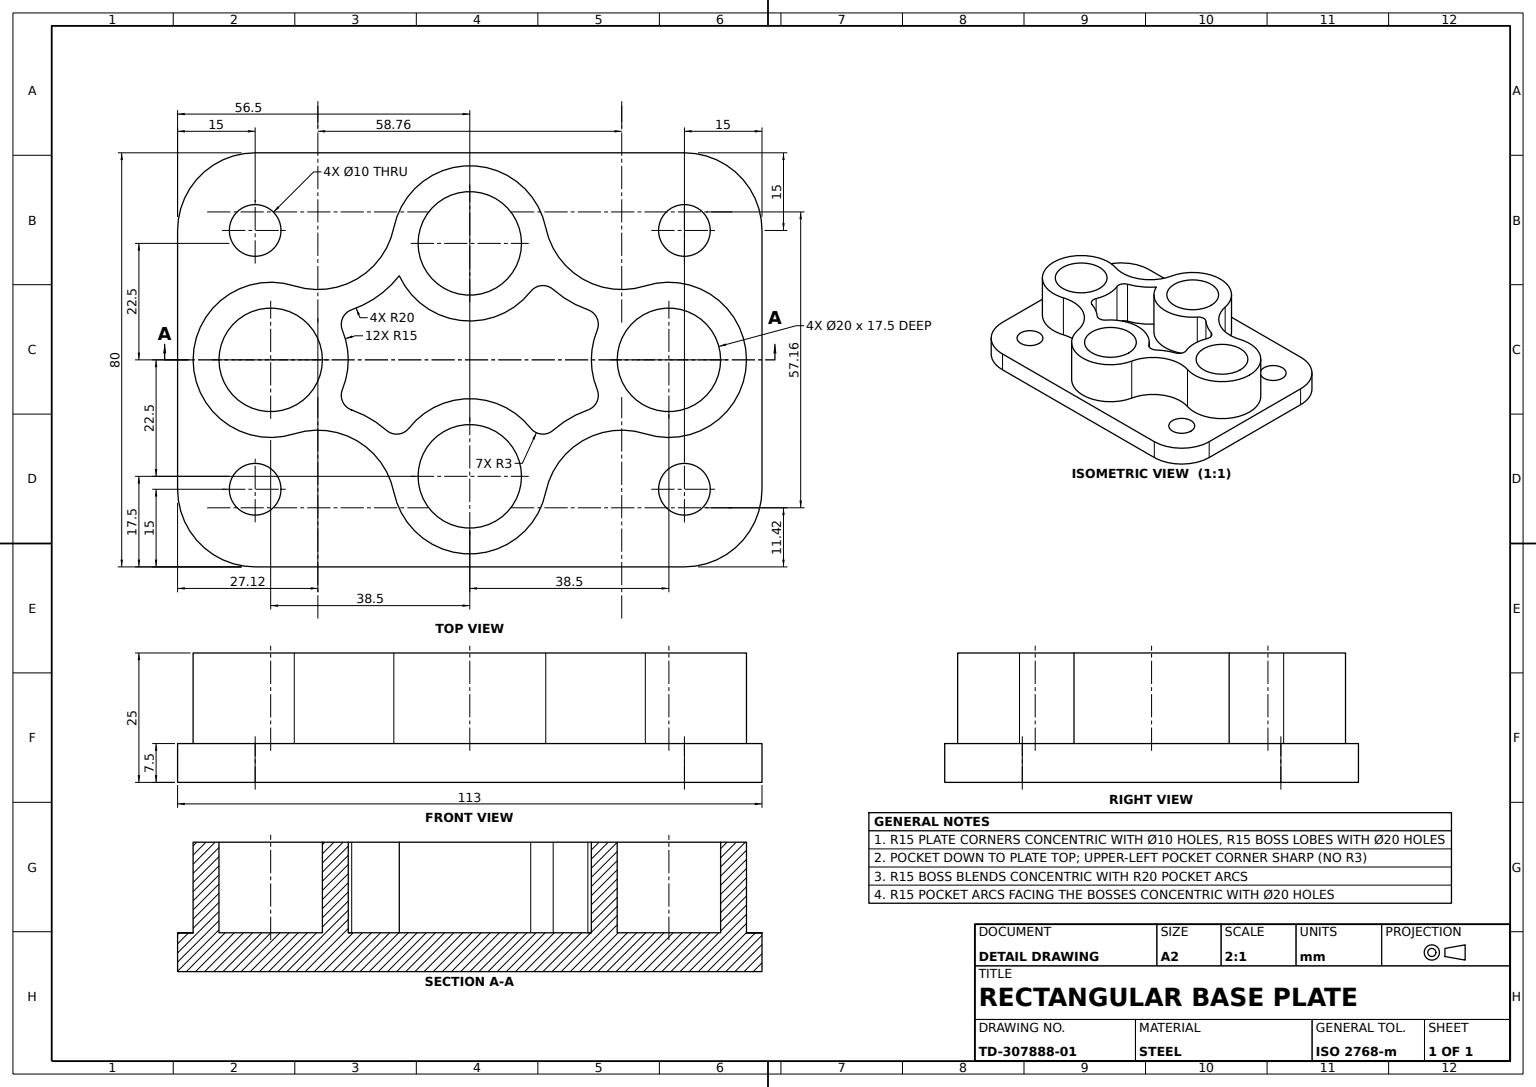
SolidWorks part; units mm, degrees
material "Plain Carbon Steel"
ref_plane "Front Plane" through (0, 0, 0) normal (0, 0, 1) x (1, 0, 0)
ref_plane "Top Plane" through (0, 0, 0) normal (0, 1, 0) x (1, 0, 0)
ref_plane "Right Plane" through (0, 0, 0) normal (1, 0, 0) x (0, 0, -1)
sketch "Base Plate Sketch" plane through (0, 0, 0) normal (0, 1, 0) x (1, 0, 0)
  line L1 (40, 0) -> (40, 56.5)
  line L2 (40, 56.5) -> (-40, 56.5)
  line L3 (-40, 56.5) -> (-40, -56.5)
  line L4 (-40, -56.5) -> (40, -56.5)
  line L5 (40, -56.5) -> (40, 0)
  dimension "D1" = 80
  dimension "D2" = 113
  dimension "D3" = 40
extrude "Base Plate" add sketch "Base Plate Sketch" along normal blind 7.5
sketch "Port Boss Sketch" plane through (0, 7.5, 0) normal (0, 1, 0) x (1, 0, 0)
  line L4 (0, -56.5) -> (0, -53.5)
  line L5 (-40, -56.5) -> (40, -56.5) construction
  circle A1 centre (0, -38.5) radius 15
  circle A2 centre (22.5, 0) radius 15
  circle A3 centre (-22.5, 0) radius 15
  circle A5 centre (0, 38.5) radius 15
  arc A6 (-25.5397, 14.6888) -> (-14.2897, 33.9388) centre (-28.5794, 29.3776) ccw
  arc A7 (14.2897, 33.9388) -> (25.5397, 14.6888) centre (28.5794, 29.3776) ccw
  arc A8 (-14.2897, -33.9388) -> (-25.5397, -14.6888) centre (-28.5794, -29.3776) ccw
  arc A9 (25.5397, -14.6888) -> (14.2897, -33.9388) centre (28.5794, -29.3776) ccw
  arc A10 (16.2452, -13.6337) -> (8.8085, -26.3588) centre (28.5794, -29.3776) ccw
  arc A11 (8.8085, 26.3588) -> (16.2452, 13.6337) centre (28.5794, 29.3776) ccw
  arc A12 (-16.2452, 13.6337) -> (-8.8085, 26.3588) centre (-28.5794, 29.3776) ccw
  arc A13 (-8.8085, -26.3588) -> (-16.2452, -13.6337) centre (-28.5794, -29.3776) ccw
  dimension "D1" = 30
  dimension "D2" = 30
  dimension "D3" = 30
  dimension "D4" = 30
  dimension "D9" = 15
  dimension "D10" = 15
  dimension "D11" = 15
  dimension "D12" = 15
  dimension "D13" = 20
  dimension "D14" = 20
  dimension "D15" = 20
  dimension "D16" = 20
  dimension "D5" = 22.5
  dimension "D6" = 22.5
  dimension "D7" = 38.5
  dimension "D8" = 38.5
extrude "Quad Port Boss" add sketch "Port Boss Sketch" along normal blind 17.5 contours A5 A11 A2 A7 | A2 | A2 A10 A1 A9 | A1 | A1 A13 A3 A8 | A3 | A3 A12 A5 A6 | A5
fillet "Boss Fillet R3 A" radius 3 1 edges at (-8.8085, 16.25, -26.3588)
fillet "Boss Fillet R3 B" radius 3 1 edges at (8.8085, 16.25, -26.3588)
fillet "Boss Fillet R3 C" radius 3 1 edges at (16.2452, 16.25, -13.6337)
fillet "Boss Fillet R3 D" radius 3 1 edges at (16.2452, 16.25, 13.6337)
fillet "Boss Fillet R3 E" radius 3 1 edges at (-16.2452, 16.25, -13.6337)
fillet "Boss Fillet R3 F" radius 3 1 edges at (-8.8085, 16.25, 26.3588)
fillet "Boss Fillet R3 G" radius 3 1 edges at (8.8085, 16.25, 26.3588)
sketch "Central Cavity Sketch" plane through (0, 25, 0) normal (0, 1, 0) x (1, 0, 0)
  circle A0 centre (0, 38.5) radius 10
  circle A1 centre (22.5, 0) radius 10
  circle A2 centre (0, -38.5) radius 10
  circle A3 centre (-22.5, 0) radius 10
  dimension "D1" = 20
extrude "Central Cavity" cut sketch "Central Cavity Sketch" against normal blind 17.5
fillet "Plate Corner Fillet R15 A" radius 15 1 edges at (-40, 3.75, -56.5)
fillet "Plate Corner Fillet R15 B" radius 15 1 edges at (40, 3.75, -56.5)
fillet "Plate Corner Fillet R15 C" radius 15 1 edges at (40, 3.75, 56.5)
fillet "Plate Corner Fillet R15 D" radius 15 1 edges at (-40, 3.75, 56.5)
sketch "Mounting Holes Sketch" plane through (0, 7.5, 0) normal (0, 1, 0) x (1, 0, 0)
  circle A0 centre (-25, 41.5) radius 5
  circle A1 centre (25, 41.5) radius 5
  circle A2 centre (25, -41.5) radius 5
  circle A3 centre (-25, -41.5) radius 5
  dimension "D1" = 10
extrude "Mounting Holes 4x" cut sketch "Mounting Holes Sketch" against normal blind 17.5
